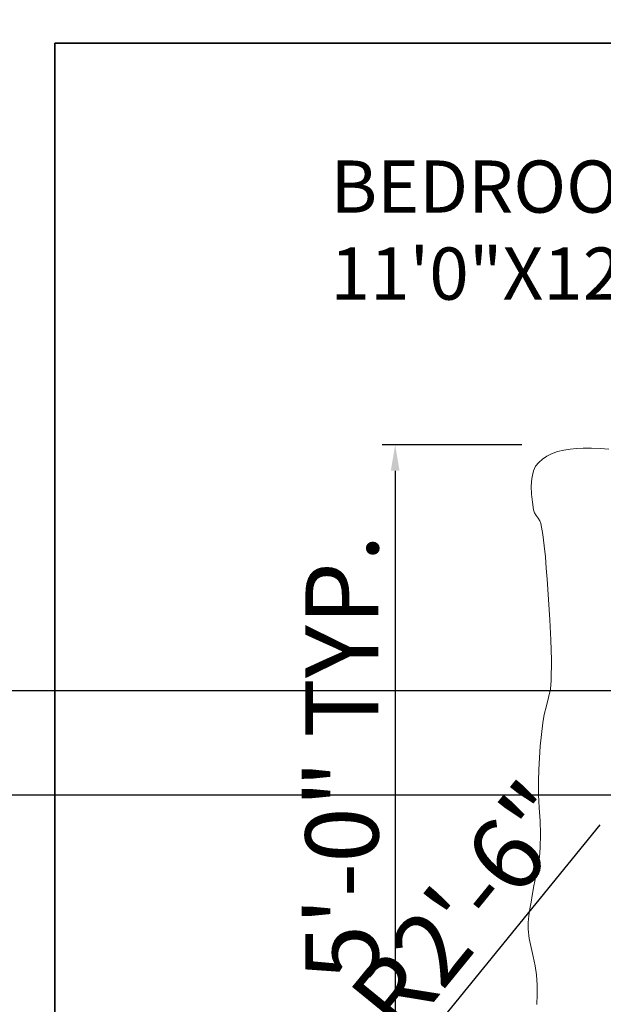
# Model space of a CAD drawing. Units: inches. Extents: x 1484 to 2008, y 1843 to 2590.
# Tile 4 of 21: x 1756 to 1811, y 1981 to 2075. Entities that reach past the tile are written whole.
import ezdxf

# ---------------------------------------------------------------- set-up
doc = ezdxf.new("R2010")
doc.units = ezdxf.units.IN
for name, color, linetype, lineweight in [('A-ANNO-DIMS', 2, 'Continuous', 18), ('A-AREA-IDEN', 7, 'Continuous', 18), ('A-FURN', 8, 'Continuous', 18), ('A-WALL', 7, 'Continuous', 35)]:
    doc.layers.add(name, color=color, linetype=linetype, lineweight=lineweight)
doc.styles.get("Standard").update_dxf_attribs({"font": 'arial.ttf'})
doc.dimstyles.new('ISO-25', dxfattribs={"dimtxt": 7, "dimasz": 2.5, "dimexe": 1.25, "dimexo": 0.625, "dimtad": 1, "dimdec": 0, "dimlunit": 3, "dimtxsty": 'Standard', "dimcen": 2.5, "dimadec": 0, "dimazin": 0, "dimtfac": 1, "dimtdec": 0, "dimtmove": 0, "dimatfit": 3, "dimfxl": 1, "dimarcsym": 0})

# ---------------------------------------------------------------- blocks, each defined once
blk = doc.blocks.new('BED-DOUBLE')
for p, q in [((0.441, 7.719), (0.376, 6.898)), ((0.376, 6.898), (0.332, 6.076)), ((0.332, 6.076), (0.338, 5.255)), ((0.338, 5.255), (0.372, 4.639)), ((0.372, 4.639), (0.426, 4.02)), ((0.426, 4.02), (0.516, 3.407)), ((0.516, 3.407), (0.66, 2.81)), ((0.66, 2.81), (0.873, 2.236)), ((0.873, 2.236), (1.095, 1.801)), ((12.88, 1.803), (14.82, 1.936)), ((14.82, 1.936), (16.762, 2.064)), ((16.762, 2.064), (18.705, 2.166)), ((18.705, 2.166), (20.649, 2.22)), ((20.649, 2.22), (22.592, 2.205)), ((22.592, 2.205), (23.412, 2.122)), ((23.412, 2.122), (24.222, 1.953)), ((24.222, 1.953), (25.027, 1.745)), ((1.095, 1.801), (1.368, 1.381)), ((1.368, 1.381), (1.693, 1.004)), ((1.693, 1.004), (2.069, 0.7)), ((6.783, 0.768), (7.028, 0.949)), ((7.028, 0.949), (7.281, 1.111)), ((7.281, 1.111), (7.555, 1.212)), ((7.555, 1.212), (8.611, 1.393)), ((8.611, 1.393), (9.673, 1.533)), ((9.673, 1.533), (10.74, 1.642)), ((10.74, 1.642), (11.81, 1.729)), ((11.81, 1.729), (12.88, 1.803)), ((25.027, 1.745), (25.834, 1.544)), ((25.834, 1.544), (26.649, 1.397)), ((26.649, 1.397), (27.761, 1.266)), ((27.761, 1.266), (28.876, 1.156)), ((28.876, 1.156), (29.992, 1.07)), ((29.992, 1.07), (31.111, 1.008)), ((31.111, 1.008), (32.229, 0.973)), ((32.229, 0.973), (33.501, 0.987)), ((33.501, 0.987), (34.773, 1.054)), ((34.773, 1.054), (36.044, 1.132)), ((36.044, 1.132), (37.315, 1.181)), ((37.315, 1.181), (38.586, 1.16)), ((38.586, 1.16), (39.513, 1.069)), ((39.513, 1.069), (40.433, 0.916)), ((2.069, 0.7), (2.497, 0.496)), ((2.497, 0.496), (3.227, 0.336)), ((3.227, 0.336), (3.978, 0.29)), ((3.978, 0.29), (4.739, 0.327)), ((4.739, 0.327), (5.501, 0.415)), ((5.501, 0.415), (6.253, 0.521)), ((6.253, 0.521), (6.529, 0.611)), ((6.529, 0.611), (6.783, 0.768)), ((40.433, 0.916), (41.349, 0.731)), ((41.349, 0.731), (42.266, 0.543)), ((42.266, 0.543), (43.186, 0.383)), ((43.186, 0.383), (43.831, 0.276)), ((43.831, 0.276), (44.478, 0.162)), ((44.478, 0.162), (45.125, 0.063)), ((45.125, 0.063), (45.774, 0.002)), ((45.774, 0.002), (46.425, 0)), ((46.425, 0), (47.304, 0.101)), ((47.304, 0.101), (48.175, 0.277)), ((48.175, 0.277), (49.042, 0.481)), ((49.042, 0.481), (49.911, 0.671)), ((49.911, 0.671), (50.789, 0.798)), ((50.789, 0.798), (51.735, 0.853)), ((51.735, 0.853), (52.684, 0.858)), ((52.684, 0.858), (53.634, 0.84))]:
    blk.add_line(p, q)
blk = doc.blocks.new('*D9')
at = {"layer": 'A-ANNO-DIMS', "color": 0, "lineweight": -2, "transparency": 16777216}
for p, q in [((1804.291, 1973.808), (1804.291, 1960.431)), ((1889.307, 1973.808), (1889.307, 1960.431)), ((1806.791, 1961.681), (1886.807, 1961.681)), ((1889.307, 1961.681), (2001.132, 1961.681))]:
    blk.add_line(p, q, dxfattribs=at)
at = {"layer": 'A-ANNO-DIMS', "color": 0, "transparency": 16777216}
for points in [[(1806.791, 1962.097), (1806.791, 1961.264), (1804.291, 1961.681)], [(1886.807, 1962.097), (1886.807, 1961.264), (1889.307, 1961.681)]]:
    blk.add_solid(points, dxfattribs=at)
at = {"layer": 'Defpoints', "color": 0, "transparency": 16777216}
for p in [(1804.291, 1974.433), (1889.307, 1974.433), (1889.307, 1961.681)]:
    blk.add_point(p, dxfattribs=at)
at = {"layer": 'A-ANNO-DIMS', "color": 0, "transparency": 16777216, "insert": (1946.47, 1965.927), "char_height": 7, "attachment_point": 5}
blk.add_mtext('DOUBLE BED 7\'-1" TYP.', dxfattribs=at)
blk = doc.blocks.new('*D10')
at = {"layer": 'A-ANNO-DIMS', "color": 0, "lineweight": -2, "transparency": 16777216}
for p, q in [((1803.666, 2034.333), (1790.288, 2034.333)), ((1791.538, 2031.833), (1791.538, 1976.933)), ((1803.666, 1974.433), (1790.288, 1974.433))]:
    blk.add_line(p, q, dxfattribs=at)
at = {"layer": 'A-ANNO-DIMS', "color": 0, "transparency": 16777216}
for points in [[(1791.122, 2031.833), (1791.955, 2031.833), (1791.538, 2034.333)], [(1791.122, 1976.933), (1791.955, 1976.933), (1791.538, 1974.433)]]:
    blk.add_solid(points, dxfattribs=at)
at = {"layer": 'Defpoints', "color": 0, "transparency": 16777216}
for p in [(1804.291, 2034.333), (1791.538, 1974.433), (1804.291, 1974.433)]:
    blk.add_point(p, dxfattribs=at)
at = {"layer": 'A-ANNO-DIMS', "color": 0, "transparency": 16777216, "insert": (1787.339, 2004.383), "char_height": 7, "attachment_point": 5, "rotation": 90}
blk.add_mtext('5\'-0" TYP.', dxfattribs=at)
blk = doc.blocks.new('*D11')
at = {"layer": 'A-ANNO-DIMS', "color": 0, "lineweight": -2, "transparency": 16777216}
for p, q in [((1754.42, 2083.338), (1754.42, 2076.976)), ((1792.67, 2083.338), (1792.67, 2076.976)), ((1756.92, 2078.226), (1790.17, 2078.226)), ((1792.67, 2078.226), (1887.105, 2078.226))]:
    blk.add_line(p, q, dxfattribs=at)
at = {"layer": 'A-ANNO-DIMS', "color": 0, "transparency": 16777216}
for points in [[(1756.92, 2078.642), (1756.92, 2077.809), (1754.42, 2078.226)], [(1790.17, 2078.642), (1790.17, 2077.809), (1792.67, 2078.226)]]:
    blk.add_solid(points, dxfattribs=at)
at = {"layer": 'Defpoints', "color": 0, "transparency": 16777216}
for p in [(1754.42, 2083.963), (1792.67, 2083.963), (1792.67, 2078.226)]:
    blk.add_point(p, dxfattribs=at)
at = {"layer": 'A-ANNO-DIMS', "color": 0, "transparency": 16777216, "insert": (1841.137, 2082.475), "char_height": 7, "attachment_point": 5}
blk.add_mtext('DOOR 3\'-2 1/2" TYP.', dxfattribs=at)
blk = doc.blocks.new('*D32')
at = {"layer": 'A-ANNO-DIMS', "color": 0, "lineweight": -2, "transparency": 16777216}
for p, q in [((1961.855, 2010.803), (1961.855, 2038.599)), ((1648.545, 2010.803), (1963.105, 2010.803)), ((1961.855, 2003.303), (1961.855, 2008.303)), ((1648.545, 2000.803), (1963.105, 2000.803))]:
    blk.add_line(p, q, dxfattribs=at)
at = {"layer": 'A-ANNO-DIMS', "color": 0, "transparency": 16777216}
for points in [[(1961.438, 2008.303), (1962.271, 2008.303), (1961.855, 2010.803)], [(1961.438, 2003.303), (1962.271, 2003.303), (1961.855, 2000.803)]]:
    blk.add_solid(points, dxfattribs=at)
at = {"layer": 'Defpoints', "color": 0, "transparency": 16777216}
for p in [(1647.92, 2010.803), (1961.855, 2010.803), (1647.92, 2000.803)]:
    blk.add_point(p, dxfattribs=at)
at = {"layer": 'A-ANNO-DIMS', "color": 0, "transparency": 16777216, "insert": (1957.656, 2025.951), "char_height": 7, "attachment_point": 5, "rotation": 90}
blk.add_mtext('0\'-10"', dxfattribs=at)
blk = doc.blocks.new('*D65')
at = {"layer": 'A-ANNO-DIMS', "color": 0, "lineweight": -2, "transparency": 16777216}
for p, q in [((1811.143, 1997.907), (1783.216, 1963.625)), ((1762.724, 1938.47), (1781.637, 1961.687))]:
    blk.add_line(p, q, dxfattribs=at)
at = {"layer": 'A-ANNO-DIMS', "color": 0, "transparency": 16777216}
blk.add_solid([(1782.893, 1963.889), (1783.539, 1963.362), (1781.637, 1961.687)], dxfattribs=at)
at = {"layer": 'Defpoints', "color": 0, "transparency": 16777216}
for p in [(1781.637, 1961.687), (1762.724, 1938.47)]:
    blk.add_point(p, dxfattribs=at)
at = {"layer": 'A-ANNO-DIMS', "color": 0, "transparency": 16777216, "insert": (1794.713, 1984.388), "char_height": 7, "attachment_point": 5, "rotation": 50.83302}
blk.add_mtext('2X R2\'-6"', dxfattribs=at)

msp = doc.modelspace()

# ---------------------------------------------------------------- linework, layer by layer
at = {"layer": 'A-WALL'}
for p, q in [((1758.92, 2072.803), (1890.92, 2072.803)), ((1758.92, 2072.803), (1758.92, 1968.173)), ((1758.92, 2060.81), (1758.92, 1968.173))]:
    msp.add_line(p, q, dxfattribs=at)

# ---------------------------------------------------------------- block references
at = {"layer": 'A-FURN', "rotation": 269.9999999999906}
msp.add_blockref('BED-DOUBLE', (1804.291, 2034.333), dxfattribs=at)

# ---------------------------------------------------------------- texts
at = {"layer": 'A-AREA-IDEN', "insert": (1785.341, 2061.564), "char_height": 5, "attachment_point": 1}
msp.add_mtext_dynamic_manual_height_columns('BEDROOM-2\\P11\'0"X12\'0"', width=40.96888, gutter_width=12.5, heights=[0], dxfattribs=at)

# ---------------------------------------------------------------- dimensions: what is measured, and where the dimension line sits
at = {"layer": 'A-ANNO-DIMS'}
for base, p1, p2, text, picture, middle in [((1792.669643705, 2078.225576395), (1754.419643705, 2083.963076395), (1792.669643705, 2083.963076395), 'DOOR <> TYP.', '*D11', (1841.137072082, 2082.474723734)), ((1889.307, 1961.681), (1804.291, 1974.433), (1889.307, 1974.433), 'DOUBLE BED <> TYP.', '*D9', (1946.47, 1965.927))]:
    dim = msp.add_linear_dim(base=base, p1=p1, p2=p2, text=text, dimstyle='ISO-25', override={"dimdec": 1, "dimlfac": 1, "dimrnd": 0, "dimzin": 1, "dimdsep": 46, "dimlunit": 4, "dimfrac": 2}, dxfattribs=at)
    dim.commit()
    dim.dimension.update_dxf_attribs({"geometry": picture, "text_midpoint": middle})
dim = msp.add_linear_dim(base=(1961.855, 2010.803), p1=(1647.92, 2000.803), p2=(1647.92, 2010.803), angle=90, dimstyle='ISO-25', override={"dimdec": 1, "dimlfac": 1, "dimrnd": 0, "dimzin": 1, "dimdsep": 46, "dimlunit": 4, "dimfrac": 2}, dxfattribs=at)
dim.commit()
dim.dimension.update_dxf_attribs({"geometry": '*D32', "text_midpoint": (1957.656, 2025.951)})
dim = msp.add_linear_dim(base=(1791.538, 1974.433), p1=(1804.291, 2034.333), p2=(1804.291, 1974.433), angle=270, text='<> TYP.', dimstyle='ISO-25', override={"dimdec": 1, "dimlfac": 1, "dimrnd": 0, "dimzin": 1, "dimdsep": 46, "dimlunit": 4, "dimfrac": 2}, dxfattribs=at)
dim.commit()
dim.dimension.update_dxf_attribs({"geometry": '*D10', "text_midpoint": (1787.339, 2004.383)})
dim = msp.add_radius_dim(center=(1762.724, 1938.47), mpoint=(1781.637, 1961.687), text='2X <>', dimstyle='ISO-25', override={"dimdec": 1, "dimlfac": 1, "dimrnd": 0, "dimzin": 1, "dimdsep": 46, "dimlunit": 4, "dimfrac": 2}, dxfattribs=at)
dim.commit()
dim.dimension.update_dxf_attribs({"geometry": '*D65', "text_midpoint": (1794.713, 1984.388)})

doc.saveas('drawing.dxf')
